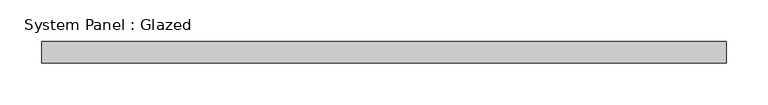
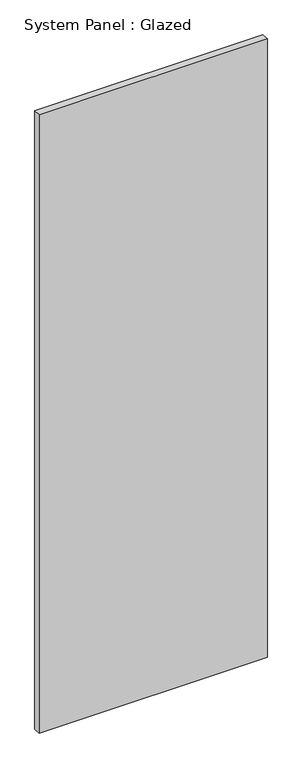
"""IFC4 building model written with IfcOpenShell, lengths in millimetres: plate geometry, System Panel : Glazed."""

from ifc_helpers import new_model, si_unit, origin, origin_with_axes, place, context, project, spatial, polyline, outline, extrude, source, transform, mapped, element, save


def system_panel_glazed_ad069301(model_context):
    return source(origin(), model_context, "Body", "SweptSolid", [
        extrude(outline(polyline([(409.5750001, 19.05), (-409.5750001, 19.05), (-409.5750001, 44.45), (409.5750001, 44.45), (409.5750001, 19.05)])), origin_with_axes(), (0.0, 0.0, 1.0), 2343.15),
    ])


if __name__ == "__main__":
    model = new_model("IFC4")
    model_context = context("Model", 3, world=origin())
    ifc_project = project(units=[si_unit("LENGTHUNIT", "METRE", prefix="MILLI")], contexts=[model_context])
    site = spatial("IfcSite", under=ifc_project)
    building = spatial("IfcBuilding", under=site)
    placement = place(None, origin())
    system_panel_glazed_shape = system_panel_glazed_ad069301(model_context)
    element("IfcPlate", 1, ObjectType="System Panel : Glazed", at=placement, inside=building, context=model_context, shape_type="MappedRepresentation", body=[
        mapped(system_panel_glazed_shape, transform((0.0, 0.0, 0.0), x_axis=(1.0, 0.0, 0.0), y_axis=(0.0, 1.0, 0.0), z_axis=(0.0, 0.0, 1.0))),
    ])
    save(model, "model.ifc")

# Revit data of these elements
# Type "System Panel : Glazed"
#   Construction Type Id = "GSP4R"
#   Analytic Construction = "1/8 in Pilkington single glazing"
#   Visual Light Transmittance = 0.9
#   Solar Heat Gain Coefficient = 0.86
#   Heat Transfer Coefficient (U) = 1.18115 BTU/(h·ft²·°F)
#   Define Thermal Properties by = 1
# Element 1 (IfcPlate, "System Panel : Glazed")
#   Materials on its faces: "Glass"
# Materials
#   "Glass": class "Glass", colour RGB 0 128 192, transparency 0.75, Description = "Soda Lime Glass", Cost = 0
